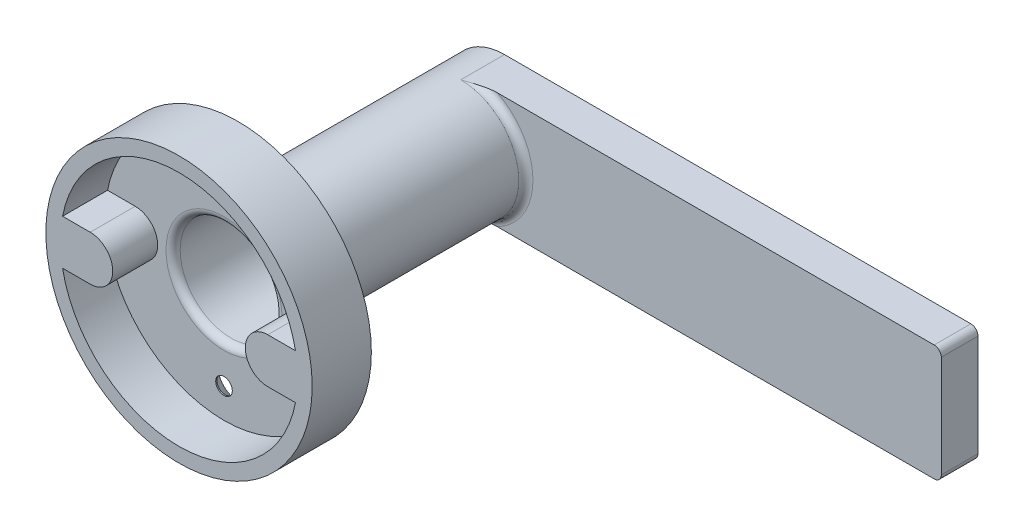
ISO-10303-21;
HEADER;
FILE_DESCRIPTION(('STEP AP214'),'2;1');
FILE_NAME('part.step','',(''),(''),'','','');
FILE_SCHEMA(('AUTOMOTIVE_DESIGN { 1 0 10303 214 1 1 1 1 }'));
ENDSEC;
DATA;
#1=APPLICATION_CONTEXT('core data for automotive mechanical design processes');
#2=APPLICATION_PROTOCOL_DEFINITION('international standard','automotive_design',2000,#1);
#3=PRODUCT_CONTEXT('',#1,'mechanical');
#4=PRODUCT('Part','Part','',(#3));
#5=PRODUCT_RELATED_PRODUCT_CATEGORY('part','',(#4));
#6=PRODUCT_DEFINITION_FORMATION('','',#4);
#7=PRODUCT_DEFINITION_CONTEXT('part definition',#1,'design');
#8=PRODUCT_DEFINITION('design','',#6,#7);
#9=PRODUCT_DEFINITION_SHAPE('','',#8);
#10=(LENGTH_UNIT() NAMED_UNIT(*) SI_UNIT(.MILLI.,.METRE.));
#11=(NAMED_UNIT(*) PLANE_ANGLE_UNIT() SI_UNIT($,.RADIAN.));
#12=(NAMED_UNIT(*) SI_UNIT($,.STERADIAN.) SOLID_ANGLE_UNIT());
#13=UNCERTAINTY_MEASURE_WITH_UNIT(LENGTH_MEASURE(1.E-05),#10,'distance_accuracy_value','');
#14=(GEOMETRIC_REPRESENTATION_CONTEXT(3) GLOBAL_UNCERTAINTY_ASSIGNED_CONTEXT((#13)) GLOBAL_UNIT_ASSIGNED_CONTEXT((#10,
#11,#12)) REPRESENTATION_CONTEXT('',''));
#15=CARTESIAN_POINT('',(0.,0.,0.));
#16=DIRECTION('',(0.,0.,1.));
#17=DIRECTION('',(1.,0.,0.));
#18=AXIS2_PLACEMENT_3D('',#15,#16,#17);
#19=CARTESIAN_POINT('',(0.,0.,12.7));
#20=DIRECTION('',(0.,0.,-1.));
#21=DIRECTION('',(-1.,0.,0.));
#22=AXIS2_PLACEMENT_3D('',#19,#20,#21);
#23=CYLINDRICAL_SURFACE('',#22,28.575);
#24=CARTESIAN_POINT('',(0.,0.,12.7));
#25=DIRECTION('',(0.,0.,1.));
#26=DIRECTION('',(1.,0.,0.));
#27=AXIS2_PLACEMENT_3D('',#24,#25,#26);
#28=CIRCLE('',#27,28.575);
#29=CARTESIAN_POINT('',(28.575,0.,12.7));
#30=VERTEX_POINT('',#29);
#31=EDGE_CURVE('E196',#30,#30,#28,.T.);
#32=ORIENTED_EDGE('',*,*,#31,.F.);
#33=EDGE_LOOP('',(#32));
#34=FACE_BOUND('',#33,.T.);
#35=CARTESIAN_POINT('',(0.,0.,0.));
#36=DIRECTION('',(0.,0.,1.));
#37=DIRECTION('',(1.,0.,0.));
#38=AXIS2_PLACEMENT_3D('',#35,#36,#37);
#39=CIRCLE('',#38,28.575);
#40=CARTESIAN_POINT('',(28.575,0.,0.));
#41=VERTEX_POINT('',#40);
#42=EDGE_CURVE('E247',#41,#41,#39,.T.);
#43=ORIENTED_EDGE('',*,*,#42,.T.);
#44=EDGE_LOOP('',(#43));
#45=FACE_BOUND('',#44,.T.);
#46=ADVANCED_FACE('F41',(#34,#45),#23,.T.);
#47=CARTESIAN_POINT('',(0.,0.,12.7));
#48=DIRECTION('',(0.,0.,1.));
#49=DIRECTION('',(1.,0.,0.));
#50=AXIS2_PLACEMENT_3D('',#47,#48,#49);
#51=PLANE('',#50);
#52=CARTESIAN_POINT('',(19.05,0.,12.7));
#53=DIRECTION('',(0.,0.,-1.));
#54=DIRECTION('',(-1.,0.,0.));
#55=AXIS2_PLACEMENT_3D('',#52,#53,#54);
#56=CIRCLE('',#55,4.826);
#57=CARTESIAN_POINT('',(19.05,-4.826,12.7));
#58=VERTEX_POINT('',#57);
#59=CARTESIAN_POINT('',(19.05,4.826,12.7));
#60=VERTEX_POINT('',#59);
#61=EDGE_CURVE('E195',#58,#60,#56,.T.);
#62=ORIENTED_EDGE('',*,*,#61,.F.);
#63=DIRECTION('',(-1.,0.,0.));
#64=VECTOR('',#63,1.);
#65=CARTESIAN_POINT('',(19.05,-4.826,12.7));
#66=LINE('',#65,#64);
#67=CARTESIAN_POINT('',(24.9900993985777,-4.826,12.7));
#68=VERTEX_POINT('',#67);
#69=EDGE_CURVE('E205',#68,#58,#66,.T.);
#70=ORIENTED_EDGE('',*,*,#69,.F.);
#71=CARTESIAN_POINT('',(0.,0.,12.7));
#72=DIRECTION('',(0.,0.,1.));
#73=DIRECTION('',(1.,0.,0.));
#74=AXIS2_PLACEMENT_3D('',#71,#72,#73);
#75=CIRCLE('',#74,25.451823980823);
#76=CARTESIAN_POINT('',(-24.9900993985777,-4.82599999999999,12.7));
#77=VERTEX_POINT('',#76);
#78=EDGE_CURVE('E241',#77,#68,#75,.T.);
#79=ORIENTED_EDGE('',*,*,#78,.F.);
#80=DIRECTION('',(-1.,0.,0.));
#81=VECTOR('',#80,1.);
#82=CARTESIAN_POINT('',(-19.05,-4.826,12.7));
#83=LINE('',#82,#81);
#84=CARTESIAN_POINT('',(-19.05,-4.826,12.7));
#85=VERTEX_POINT('',#84);
#86=EDGE_CURVE('E238',#85,#77,#83,.T.);
#87=ORIENTED_EDGE('',*,*,#86,.F.);
#88=CARTESIAN_POINT('',(-19.05,0.,12.7));
#89=DIRECTION('',(0.,0.,-1.));
#90=DIRECTION('',(1.,0.,0.));
#91=AXIS2_PLACEMENT_3D('',#88,#89,#90);
#92=CIRCLE('',#91,4.826);
#93=CARTESIAN_POINT('',(-19.05,4.826,12.7));
#94=VERTEX_POINT('',#93);
#95=EDGE_CURVE('E232',#94,#85,#92,.T.);
#96=ORIENTED_EDGE('',*,*,#95,.F.);
#97=DIRECTION('',(1.,0.,0.));
#98=VECTOR('',#97,1.);
#99=CARTESIAN_POINT('',(-19.05,4.826,12.7));
#100=LINE('',#99,#98);
#101=CARTESIAN_POINT('',(-24.9900993985777,4.826,12.7));
#102=VERTEX_POINT('',#101);
#103=EDGE_CURVE('E235',#102,#94,#100,.T.);
#104=ORIENTED_EDGE('',*,*,#103,.F.);
#105=CARTESIAN_POINT('',(0.,0.,12.7));
#106=DIRECTION('',(0.,0.,1.));
#107=DIRECTION('',(1.,0.,0.));
#108=AXIS2_PLACEMENT_3D('',#105,#106,#107);
#109=CIRCLE('',#108,25.451823980823);
#110=CARTESIAN_POINT('',(24.9900993985777,4.826,12.7));
#111=VERTEX_POINT('',#110);
#112=EDGE_CURVE('E230',#111,#102,#109,.T.);
#113=ORIENTED_EDGE('',*,*,#112,.F.);
#114=DIRECTION('',(1.,0.,0.));
#115=VECTOR('',#114,1.);
#116=CARTESIAN_POINT('',(19.05,4.826,12.7));
#117=LINE('',#116,#115);
#118=EDGE_CURVE('E228',#60,#111,#117,.T.);
#119=ORIENTED_EDGE('',*,*,#118,.F.);
#120=EDGE_LOOP('',(#62,#70,#79,#87,#96,#104,#113,#119));
#121=FACE_BOUND('',#120,.T.);
#122=ORIENTED_EDGE('',*,*,#31,.T.);
#123=EDGE_LOOP('',(#122));
#124=FACE_BOUND('',#123,.T.);
#125=ADVANCED_FACE('F342',(#121,#124),#51,.T.);
#126=CARTESIAN_POINT('',(0.,0.,0.));
#127=DIRECTION('',(0.,0.,1.));
#128=DIRECTION('',(1.,0.,0.));
#129=AXIS2_PLACEMENT_3D('',#126,#127,#128);
#130=PLANE('',#129);
#131=CARTESIAN_POINT('',(0.,-19.05,0.));
#132=DIRECTION('',(0.,0.,1.));
#133=DIRECTION('',(1.,0.,0.));
#134=AXIS2_PLACEMENT_3D('',#131,#132,#133);
#135=CIRCLE('',#134,4.37800000000003);
#136=CARTESIAN_POINT('',(4.37800000000003,-19.05,0.));
#137=VERTEX_POINT('',#136);
#138=EDGE_CURVE('E49',#137,#137,#135,.T.);
#139=ORIENTED_EDGE('',*,*,#138,.T.);
#140=EDGE_LOOP('',(#139));
#141=FACE_BOUND('',#140,.T.);
#142=CARTESIAN_POINT('',(0.,19.05,0.));
#143=DIRECTION('',(0.,0.,1.));
#144=DIRECTION('',(1.,0.,0.));
#145=AXIS2_PLACEMENT_3D('',#142,#143,#144);
#146=CIRCLE('',#145,4.37800000000003);
#147=CARTESIAN_POINT('',(4.37800000000003,19.05,0.));
#148=VERTEX_POINT('',#147);
#149=EDGE_CURVE('E425',#148,#148,#146,.T.);
#150=ORIENTED_EDGE('',*,*,#149,.T.);
#151=EDGE_LOOP('',(#150));
#152=FACE_BOUND('',#151,.T.);
#153=CARTESIAN_POINT('',(0.,0.,0.));
#154=DIRECTION('',(0.,0.,-1.));
#155=DIRECTION('',(-1.,0.,0.));
#156=AXIS2_PLACEMENT_3D('',#153,#154,#155);
#157=CIRCLE('',#156,12.446);
#158=CARTESIAN_POINT('',(-12.446,0.,0.));
#159=VERTEX_POINT('',#158);
#160=EDGE_CURVE('E193',#159,#159,#157,.T.);
#161=ORIENTED_EDGE('',*,*,#160,.F.);
#162=EDGE_LOOP('',(#161));
#163=FACE_BOUND('',#162,.T.);
#164=ORIENTED_EDGE('',*,*,#42,.F.);
#165=EDGE_LOOP('',(#164));
#166=FACE_BOUND('',#165,.T.);
#167=ADVANCED_FACE('F349',(#141,#152,#163,#166),#130,.F.);
#168=CARTESIAN_POINT('',(19.05,0.,3.048));
#169=DIRECTION('',(0.,0.,1.));
#170=DIRECTION('',(1.,0.,0.));
#171=AXIS2_PLACEMENT_3D('',#168,#169,#170);
#172=CYLINDRICAL_SURFACE('',#171,4.826);
#173=ORIENTED_EDGE('',*,*,#61,.T.);
#174=DIRECTION('',(0.,0.,1.));
#175=VECTOR('',#174,1.);
#176=CARTESIAN_POINT('',(19.05,4.826,3.048));
#177=LINE('',#176,#175);
#178=CARTESIAN_POINT('',(19.05,4.826,3.048));
#179=VERTEX_POINT('',#178);
#180=EDGE_CURVE('E221',#179,#60,#177,.T.);
#181=ORIENTED_EDGE('',*,*,#180,.F.);
#182=CARTESIAN_POINT('',(19.05,0.,3.048));
#183=DIRECTION('',(0.,0.,-1.));
#184=DIRECTION('',(-1.,0.,0.));
#185=AXIS2_PLACEMENT_3D('',#182,#183,#184);
#186=CIRCLE('',#185,4.826);
#187=CARTESIAN_POINT('',(19.05,-4.826,3.048));
#188=VERTEX_POINT('',#187);
#189=EDGE_CURVE('E197',#188,#179,#186,.T.);
#190=ORIENTED_EDGE('',*,*,#189,.F.);
#191=DIRECTION('',(0.,0.,1.));
#192=VECTOR('',#191,1.);
#193=CARTESIAN_POINT('',(19.05,-4.826,3.048));
#194=LINE('',#193,#192);
#195=EDGE_CURVE('E246',#188,#58,#194,.T.);
#196=ORIENTED_EDGE('',*,*,#195,.T.);
#197=EDGE_LOOP('',(#173,#181,#190,#196));
#198=FACE_BOUND('',#197,.T.);
#199=ADVANCED_FACE('F356',(#198),#172,.T.);
#200=CARTESIAN_POINT('',(19.05,-4.826,3.048));
#201=DIRECTION('',(0.,1.,0.));
#202=DIRECTION('',(-1.,0.,0.));
#203=AXIS2_PLACEMENT_3D('',#200,#201,#202);
#204=PLANE('',#203);
#205=ORIENTED_EDGE('',*,*,#69,.T.);
#206=ORIENTED_EDGE('',*,*,#195,.F.);
#207=DIRECTION('',(-1.,0.,0.));
#208=VECTOR('',#207,1.);
#209=CARTESIAN_POINT('',(19.05,-4.826,3.048));
#210=LINE('',#209,#208);
#211=CARTESIAN_POINT('',(24.9900993985777,-4.826,3.048));
#212=VERTEX_POINT('',#211);
#213=EDGE_CURVE('E222',#212,#188,#210,.T.);
#214=ORIENTED_EDGE('',*,*,#213,.F.);
#215=DIRECTION('',(0.,0.,1.));
#216=VECTOR('',#215,1.);
#217=CARTESIAN_POINT('',(24.9900993985777,-4.826,3.048));
#218=LINE('',#217,#216);
#219=EDGE_CURVE('E248',#212,#68,#218,.T.);
#220=ORIENTED_EDGE('',*,*,#219,.T.);
#221=EDGE_LOOP('',(#205,#206,#214,#220));
#222=FACE_BOUND('',#221,.T.);
#223=ADVANCED_FACE('F362',(#222),#204,.F.);
#224=CARTESIAN_POINT('',(0.,0.,3.048));
#225=DIRECTION('',(0.,0.,1.));
#226=DIRECTION('',(1.,0.,0.));
#227=AXIS2_PLACEMENT_3D('',#224,#225,#226);
#228=CYLINDRICAL_SURFACE('',#227,25.451823980823);
#229=ORIENTED_EDGE('',*,*,#78,.T.);
#230=ORIENTED_EDGE('',*,*,#219,.F.);
#231=CARTESIAN_POINT('',(0.,0.,3.048));
#232=DIRECTION('',(0.,0.,1.));
#233=DIRECTION('',(1.,0.,0.));
#234=AXIS2_PLACEMENT_3D('',#231,#232,#233);
#235=CIRCLE('',#234,25.451823980823);
#236=CARTESIAN_POINT('',(-24.9900993985777,-4.82599999999999,3.048));
#237=VERTEX_POINT('',#236);
#238=EDGE_CURVE('E216',#237,#212,#235,.T.);
#239=ORIENTED_EDGE('',*,*,#238,.F.);
#240=DIRECTION('',(0.,0.,1.));
#241=VECTOR('',#240,1.);
#242=CARTESIAN_POINT('',(-24.9900993985777,-4.82599999999999,3.048));
#243=LINE('',#242,#241);
#244=EDGE_CURVE('E252',#237,#77,#243,.T.);
#245=ORIENTED_EDGE('',*,*,#244,.T.);
#246=EDGE_LOOP('',(#229,#230,#239,#245));
#247=FACE_BOUND('',#246,.T.);
#248=ADVANCED_FACE('F393',(#247),#228,.F.);
#249=CARTESIAN_POINT('',(-19.05,-4.826,3.048));
#250=DIRECTION('',(0.,1.,0.));
#251=DIRECTION('',(-1.,0.,0.));
#252=AXIS2_PLACEMENT_3D('',#249,#250,#251);
#253=PLANE('',#252);
#254=ORIENTED_EDGE('',*,*,#86,.T.);
#255=ORIENTED_EDGE('',*,*,#244,.F.);
#256=DIRECTION('',(-1.,0.,0.));
#257=VECTOR('',#256,1.);
#258=CARTESIAN_POINT('',(-19.05,-4.826,3.048));
#259=LINE('',#258,#257);
#260=CARTESIAN_POINT('',(-19.05,-4.826,3.048));
#261=VERTEX_POINT('',#260);
#262=EDGE_CURVE('E212',#261,#237,#259,.T.);
#263=ORIENTED_EDGE('',*,*,#262,.F.);
#264=DIRECTION('',(0.,0.,1.));
#265=VECTOR('',#264,1.);
#266=CARTESIAN_POINT('',(-19.05,-4.826,3.048));
#267=LINE('',#266,#265);
#268=EDGE_CURVE('E254',#261,#85,#267,.T.);
#269=ORIENTED_EDGE('',*,*,#268,.T.);
#270=EDGE_LOOP('',(#254,#255,#263,#269));
#271=FACE_BOUND('',#270,.T.);
#272=ADVANCED_FACE('F386',(#271),#253,.F.);
#273=CARTESIAN_POINT('',(-19.05,0.,3.048));
#274=DIRECTION('',(0.,0.,1.));
#275=DIRECTION('',(1.,0.,0.));
#276=AXIS2_PLACEMENT_3D('',#273,#274,#275);
#277=CYLINDRICAL_SURFACE('',#276,4.826);
#278=ORIENTED_EDGE('',*,*,#95,.T.);
#279=ORIENTED_EDGE('',*,*,#268,.F.);
#280=CARTESIAN_POINT('',(-19.05,0.,3.048));
#281=DIRECTION('',(0.,0.,-1.));
#282=DIRECTION('',(1.,0.,0.));
#283=AXIS2_PLACEMENT_3D('',#280,#281,#282);
#284=CIRCLE('',#283,4.826);
#285=CARTESIAN_POINT('',(-19.05,4.826,3.048));
#286=VERTEX_POINT('',#285);
#287=EDGE_CURVE('E211',#286,#261,#284,.T.);
#288=ORIENTED_EDGE('',*,*,#287,.F.);
#289=DIRECTION('',(0.,0.,1.));
#290=VECTOR('',#289,1.);
#291=CARTESIAN_POINT('',(-19.05,4.826,3.048));
#292=LINE('',#291,#290);
#293=EDGE_CURVE('E253',#286,#94,#292,.T.);
#294=ORIENTED_EDGE('',*,*,#293,.T.);
#295=EDGE_LOOP('',(#278,#279,#288,#294));
#296=FACE_BOUND('',#295,.T.);
#297=ADVANCED_FACE('F384',(#296),#277,.T.);
#298=CARTESIAN_POINT('',(-19.05,4.826,3.048));
#299=DIRECTION('',(0.,-1.,0.));
#300=DIRECTION('',(1.,0.,0.));
#301=AXIS2_PLACEMENT_3D('',#298,#299,#300);
#302=PLANE('',#301);
#303=ORIENTED_EDGE('',*,*,#103,.T.);
#304=ORIENTED_EDGE('',*,*,#293,.F.);
#305=DIRECTION('',(1.,0.,0.));
#306=VECTOR('',#305,1.);
#307=CARTESIAN_POINT('',(-19.05,4.826,3.048));
#308=LINE('',#307,#306);
#309=CARTESIAN_POINT('',(-24.9900993985777,4.826,3.048));
#310=VERTEX_POINT('',#309);
#311=EDGE_CURVE('E209',#310,#286,#308,.T.);
#312=ORIENTED_EDGE('',*,*,#311,.F.);
#313=DIRECTION('',(0.,0.,1.));
#314=VECTOR('',#313,1.);
#315=CARTESIAN_POINT('',(-24.9900993985777,4.826,3.048));
#316=LINE('',#315,#314);
#317=EDGE_CURVE('E256',#310,#102,#316,.T.);
#318=ORIENTED_EDGE('',*,*,#317,.T.);
#319=EDGE_LOOP('',(#303,#304,#312,#318));
#320=FACE_BOUND('',#319,.T.);
#321=ADVANCED_FACE('F378',(#320),#302,.F.);
#322=CARTESIAN_POINT('',(0.,0.,3.048));
#323=DIRECTION('',(0.,0.,1.));
#324=DIRECTION('',(1.,0.,0.));
#325=AXIS2_PLACEMENT_3D('',#322,#323,#324);
#326=CYLINDRICAL_SURFACE('',#325,25.451823980823);
#327=ORIENTED_EDGE('',*,*,#112,.T.);
#328=ORIENTED_EDGE('',*,*,#317,.F.);
#329=CARTESIAN_POINT('',(0.,0.,3.048));
#330=DIRECTION('',(0.,0.,1.));
#331=DIRECTION('',(1.,0.,0.));
#332=AXIS2_PLACEMENT_3D('',#329,#330,#331);
#333=CIRCLE('',#332,25.451823980823);
#334=CARTESIAN_POINT('',(24.9900993985777,4.826,3.048));
#335=VERTEX_POINT('',#334);
#336=EDGE_CURVE('E207',#335,#310,#333,.T.);
#337=ORIENTED_EDGE('',*,*,#336,.F.);
#338=DIRECTION('',(0.,0.,1.));
#339=VECTOR('',#338,1.);
#340=CARTESIAN_POINT('',(24.9900993985777,4.826,3.048));
#341=LINE('',#340,#339);
#342=EDGE_CURVE('E258',#335,#111,#341,.T.);
#343=ORIENTED_EDGE('',*,*,#342,.T.);
#344=EDGE_LOOP('',(#327,#328,#337,#343));
#345=FACE_BOUND('',#344,.T.);
#346=ADVANCED_FACE('F374',(#345),#326,.F.);
#347=CARTESIAN_POINT('',(19.05,4.826,3.048));
#348=DIRECTION('',(0.,-1.,0.));
#349=DIRECTION('',(1.,0.,0.));
#350=AXIS2_PLACEMENT_3D('',#347,#348,#349);
#351=PLANE('',#350);
#352=ORIENTED_EDGE('',*,*,#118,.T.);
#353=ORIENTED_EDGE('',*,*,#342,.F.);
#354=DIRECTION('',(1.,0.,0.));
#355=VECTOR('',#354,1.);
#356=CARTESIAN_POINT('',(19.05,4.826,3.048));
#357=LINE('',#356,#355);
#358=EDGE_CURVE('E204',#179,#335,#357,.T.);
#359=ORIENTED_EDGE('',*,*,#358,.F.);
#360=ORIENTED_EDGE('',*,*,#180,.T.);
#361=EDGE_LOOP('',(#352,#353,#359,#360));
#362=FACE_BOUND('',#361,.T.);
#363=ADVANCED_FACE('F371',(#362),#351,.F.);
#364=CARTESIAN_POINT('',(19.05,0.,3.048));
#365=DIRECTION('',(0.,0.,-1.));
#366=DIRECTION('',(-1.,0.,0.));
#367=AXIS2_PLACEMENT_3D('',#364,#365,#366);
#368=PLANE('',#367);
#369=CARTESIAN_POINT('',(0.,19.05,3.048));
#370=DIRECTION('',(0.,0.,1.));
#371=DIRECTION('',(1.,0.,0.));
#372=AXIS2_PLACEMENT_3D('',#369,#370,#371);
#373=CIRCLE('',#372,1.778);
#374=CARTESIAN_POINT('',(1.778,19.05,3.048));
#375=VERTEX_POINT('',#374);
#376=EDGE_CURVE('E187',#375,#375,#373,.T.);
#377=ORIENTED_EDGE('',*,*,#376,.F.);
#378=EDGE_LOOP('',(#377));
#379=FACE_BOUND('',#378,.T.);
#380=CARTESIAN_POINT('',(0.,-19.05,3.048));
#381=DIRECTION('',(0.,0.,1.));
#382=DIRECTION('',(-1.,0.,0.));
#383=AXIS2_PLACEMENT_3D('',#380,#381,#382);
#384=CIRCLE('',#383,1.778);
#385=CARTESIAN_POINT('',(-1.778,-19.05,3.048));
#386=VERTEX_POINT('',#385);
#387=EDGE_CURVE('E436',#386,#386,#384,.T.);
#388=ORIENTED_EDGE('',*,*,#387,.F.);
#389=EDGE_LOOP('',(#388));
#390=FACE_BOUND('',#389,.T.);
#391=CARTESIAN_POINT('',(0.,0.,3.048));
#392=DIRECTION('',(0.,0.,-1.));
#393=DIRECTION('',(-1.,0.,0.));
#394=AXIS2_PLACEMENT_3D('',#391,#392,#393);
#395=CIRCLE('',#394,12.446);
#396=CARTESIAN_POINT('',(-12.446,0.,3.048));
#397=VERTEX_POINT('',#396);
#398=EDGE_CURVE('E280',#397,#397,#395,.T.);
#399=ORIENTED_EDGE('',*,*,#398,.T.);
#400=EDGE_LOOP('',(#399));
#401=FACE_BOUND('',#400,.T.);
#402=ORIENTED_EDGE('',*,*,#189,.T.);
#403=ORIENTED_EDGE('',*,*,#358,.T.);
#404=ORIENTED_EDGE('',*,*,#336,.T.);
#405=ORIENTED_EDGE('',*,*,#311,.T.);
#406=ORIENTED_EDGE('',*,*,#287,.T.);
#407=ORIENTED_EDGE('',*,*,#262,.T.);
#408=ORIENTED_EDGE('',*,*,#238,.T.);
#409=ORIENTED_EDGE('',*,*,#213,.T.);
#410=EDGE_LOOP('',(#402,#403,#404,#405,#406,#407,#408,#409));
#411=FACE_BOUND('',#410,.T.);
#412=ADVANCED_FACE('F372',(#379,#390,#401,#411),#368,.F.);
#413=CARTESIAN_POINT('',(0.,0.,-49.276));
#414=DIRECTION('',(0.,0.,1.));
#415=DIRECTION('',(1.,0.,0.));
#416=AXIS2_PLACEMENT_3D('',#413,#414,#415);
#417=CYLINDRICAL_SURFACE('',#416,12.446);
#418=DIRECTION('',(0.,0.,1.));
#419=VECTOR('',#418,1.);
#420=CARTESIAN_POINT('',(0.,-12.446,-57.15));
#421=LINE('',#420,#419);
#422=CARTESIAN_POINT('',(0.,-12.446,-57.15));
#423=VERTEX_POINT('',#422);
#424=CARTESIAN_POINT('',(0.,-12.446,-47.752));
#425=VERTEX_POINT('',#424);
#426=EDGE_CURVE('E168',#423,#425,#421,.T.);
#427=ORIENTED_EDGE('',*,*,#426,.T.);
#428=CARTESIAN_POINT('',(0.,0.,-47.752));
#429=DIRECTION('',(0.,0.,-1.));
#430=DIRECTION('',(-1.,0.,0.));
#431=AXIS2_PLACEMENT_3D('',#428,#429,#430);
#432=CIRCLE('',#431,12.446);
#433=CARTESIAN_POINT('',(0.,12.446,-47.752));
#434=VERTEX_POINT('',#433);
#435=EDGE_CURVE('E271',#425,#434,#432,.F.);
#436=ORIENTED_EDGE('',*,*,#435,.T.);
#437=DIRECTION('',(0.,0.,1.));
#438=VECTOR('',#437,1.);
#439=CARTESIAN_POINT('',(0.,12.446,-57.15));
#440=LINE('',#439,#438);
#441=CARTESIAN_POINT('',(0.,12.446,-57.15));
#442=VERTEX_POINT('',#441);
#443=EDGE_CURVE('E172',#442,#434,#440,.T.);
#444=ORIENTED_EDGE('',*,*,#443,.F.);
#445=CARTESIAN_POINT('',(0.,0.,-57.15));
#446=DIRECTION('',(0.,0.,-1.));
#447=DIRECTION('',(-1.,0.,0.));
#448=AXIS2_PLACEMENT_3D('',#445,#446,#447);
#449=CIRCLE('',#448,12.446);
#450=EDGE_CURVE('E157',#423,#442,#449,.T.);
#451=ORIENTED_EDGE('',*,*,#450,.F.);
#452=EDGE_LOOP('',(#427,#436,#444,#451));
#453=FACE_BOUND('',#452,.T.);
#454=ORIENTED_EDGE('',*,*,#160,.T.);
#455=EDGE_LOOP('',(#454));
#456=FACE_BOUND('',#455,.T.);
#457=ADVANCED_FACE('F176',(#453,#456),#417,.T.);
#458=CARTESIAN_POINT('',(0.,0.,-80.1680810564779));
#459=DIRECTION('',(0.,0.,1.));
#460=DIRECTION('',(1.,0.,0.));
#461=AXIS2_PLACEMENT_3D('',#458,#459,#460);
#462=CYLINDRICAL_SURFACE('',#461,10.922);
#463=CARTESIAN_POINT('',(0.,0.,1.524));
#464=DIRECTION('',(0.,0.,-1.));
#465=DIRECTION('',(-1.,0.,0.));
#466=AXIS2_PLACEMENT_3D('',#463,#464,#465);
#467=CIRCLE('',#466,10.922);
#468=CARTESIAN_POINT('',(-10.922,0.,1.524));
#469=VERTEX_POINT('',#468);
#470=EDGE_CURVE('E273',#469,#469,#467,.F.);
#471=ORIENTED_EDGE('',*,*,#470,.T.);
#472=EDGE_LOOP('',(#471));
#473=FACE_BOUND('',#472,.T.);
#474=CARTESIAN_POINT('',(0.,0.,-49.276));
#475=DIRECTION('',(0.,0.,-1.));
#476=DIRECTION('',(-1.,0.,0.));
#477=AXIS2_PLACEMENT_3D('',#474,#475,#476);
#478=CIRCLE('',#477,10.922);
#479=CARTESIAN_POINT('',(-10.922,0.,-49.276));
#480=VERTEX_POINT('',#479);
#481=EDGE_CURVE('E173',#480,#480,#478,.F.);
#482=ORIENTED_EDGE('',*,*,#481,.F.);
#483=EDGE_LOOP('',(#482));
#484=FACE_BOUND('',#483,.T.);
#485=ADVANCED_FACE('F401',(#473,#484),#462,.F.);
#486=CARTESIAN_POINT('',(0.,0.,-57.15));
#487=DIRECTION('',(0.,0.,-1.));
#488=DIRECTION('',(-1.,0.,0.));
#489=AXIS2_PLACEMENT_3D('',#486,#487,#488);
#490=PLANE('',#489);
#491=DIRECTION('',(0.,-1.,0.));
#492=VECTOR('',#491,1.);
#493=CARTESIAN_POINT('',(101.6,12.446,-57.15));
#494=LINE('',#493,#492);
#495=CARTESIAN_POINT('',(101.6,10.922,-57.15));
#496=VERTEX_POINT('',#495);
#497=CARTESIAN_POINT('',(101.6,-10.922,-57.15));
#498=VERTEX_POINT('',#497);
#499=EDGE_CURVE('E161',#496,#498,#494,.T.);
#500=ORIENTED_EDGE('',*,*,#499,.T.);
#501=CARTESIAN_POINT('',(100.076,-10.922,-57.15));
#502=DIRECTION('',(0.,0.,-1.));
#503=DIRECTION('',(-1.,0.,0.));
#504=AXIS2_PLACEMENT_3D('',#501,#502,#503);
#505=CIRCLE('',#504,1.524);
#506=CARTESIAN_POINT('',(100.076,-12.446,-57.15));
#507=VERTEX_POINT('',#506);
#508=EDGE_CURVE('E156',#498,#507,#505,.T.);
#509=ORIENTED_EDGE('',*,*,#508,.T.);
#510=DIRECTION('',(-1.,0.,0.));
#511=VECTOR('',#510,1.);
#512=CARTESIAN_POINT('',(101.6,-12.446,-57.15));
#513=LINE('',#512,#511);
#514=EDGE_CURVE('E155',#507,#423,#513,.T.);
#515=ORIENTED_EDGE('',*,*,#514,.T.);
#516=ORIENTED_EDGE('',*,*,#450,.T.);
#517=DIRECTION('',(1.,0.,0.));
#518=VECTOR('',#517,1.);
#519=CARTESIAN_POINT('',(101.6,12.446,-57.15));
#520=LINE('',#519,#518);
#521=CARTESIAN_POINT('',(100.076,12.446,-57.15));
#522=VERTEX_POINT('',#521);
#523=EDGE_CURVE('E178',#442,#522,#520,.T.);
#524=ORIENTED_EDGE('',*,*,#523,.T.);
#525=CARTESIAN_POINT('',(100.076,10.922,-57.15));
#526=DIRECTION('',(0.,0.,-1.));
#527=DIRECTION('',(-1.,0.,0.));
#528=AXIS2_PLACEMENT_3D('',#525,#526,#527);
#529=CIRCLE('',#528,1.524);
#530=EDGE_CURVE('E289',#522,#496,#529,.T.);
#531=ORIENTED_EDGE('',*,*,#530,.T.);
#532=EDGE_LOOP('',(#500,#509,#515,#516,#524,#531));
#533=FACE_BOUND('',#532,.T.);
#534=ADVANCED_FACE('F152',(#533),#490,.T.);
#535=CARTESIAN_POINT('',(101.6,12.446,-57.15));
#536=DIRECTION('',(0.,-1.,0.));
#537=DIRECTION('',(0.,0.,-1.));
#538=AXIS2_PLACEMENT_3D('',#535,#536,#537);
#539=PLANE('',#538);
#540=DIRECTION('',(1.,0.,0.));
#541=VECTOR('',#540,1.);
#542=CARTESIAN_POINT('',(101.6,12.446,-49.276));
#543=LINE('',#542,#541);
#544=CARTESIAN_POINT('',(6.34491796637277,12.446,-49.276));
#545=VERTEX_POINT('',#544);
#546=CARTESIAN_POINT('',(100.076,12.446,-49.276));
#547=VERTEX_POINT('',#546);
#548=EDGE_CURVE('E189',#545,#547,#543,.T.);
#549=ORIENTED_EDGE('',*,*,#548,.T.);
#550=DIRECTION('',(0.,0.,1.));
#551=VECTOR('',#550,1.);
#552=CARTESIAN_POINT('',(100.076,12.446,-57.15));
#553=LINE('',#552,#551);
#554=EDGE_CURVE('E60',#547,#522,#553,.F.);
#555=ORIENTED_EDGE('',*,*,#554,.T.);
#556=ORIENTED_EDGE('',*,*,#523,.F.);
#557=ORIENTED_EDGE('',*,*,#443,.T.);
#558=CARTESIAN_POINT('',(6.34491796637277,12.446,-49.276));
#559=CARTESIAN_POINT('',(6.21533524094485,12.446,-49.2759732705405));
#560=CARTESIAN_POINT('',(6.08579369063811,12.446,-49.27259226928));
#561=CARTESIAN_POINT('',(5.82706524459241,12.446,-49.259910087951));
#562=CARTESIAN_POINT('',(5.6978781945778,12.446,-49.2506121205866));
#563=CARTESIAN_POINT('',(5.4402955593906,12.446,-49.2269107528351));
#564=CARTESIAN_POINT('',(5.31189882415412,12.446,-49.2125195023357));
#565=CARTESIAN_POINT('',(5.05567590714475,12.446,-49.1792496205522));
#566=CARTESIAN_POINT('',(4.92784981517291,12.446,-49.1603703067066));
#567=CARTESIAN_POINT('',(4.54726190236325,12.446,-49.0981575716032));
#568=CARTESIAN_POINT('',(4.29543863295937,12.446,-49.0490520465874));
#569=CARTESIAN_POINT('',(3.79431096207436,12.446,-48.9389015359754));
#570=CARTESIAN_POINT('',(3.54500841851374,12.446,-48.8778483354951));
#571=CARTESIAN_POINT('',(3.01979635859548,12.446,-48.7389881468602));
#572=CARTESIAN_POINT('',(2.74418711385954,12.446,-48.6600566773526));
#573=CARTESIAN_POINT('',(2.19547772469525,12.446,-48.4941969315973));
#574=CARTESIAN_POINT('',(1.92237711929461,12.446,-48.4072701582111));
#575=CARTESIAN_POINT('',(1.1047936535399,12.446,-48.1385183371954));
#576=CARTESIAN_POINT('',(0.562885676700975,12.446,-47.9489679517187));
#577=CARTESIAN_POINT('',(0.0140400977837042,12.446,-47.7569129993086));
#578=CARTESIAN_POINT('',(0.00702004561032453,12.446,-47.7544564925513));
#579=CARTESIAN_POINT('',(0.,12.446,-47.752));
#580=B_SPLINE_CURVE_WITH_KNOTS('',3,(#558,#559,#560,#561,#562,#563,#564,#565,#566,#567,#568,
#569,#570,#571,#572,#573,#574,#575,#576,#577,#578,#579),.UNSPECIFIED.,.F.,.F.,(4,2,2,2,2,2,2,2,
2,2,4),(0.,0.388645930924585,0.777081020636638,1.16459568621553,1.5521693242234,
2.32144242636155,3.09124632924267,3.95113147757733,4.81085532404043,6.5329742853189,
6.5552866137498),.UNSPECIFIED.);
#581=EDGE_CURVE('E296',#434,#545,#580,.F.);
#582=ORIENTED_EDGE('',*,*,#581,.T.);
#583=EDGE_LOOP('',(#549,#555,#556,#557,#582));
#584=FACE_BOUND('',#583,.T.);
#585=ADVANCED_FACE('F414',(#584),#539,.F.);
#586=CARTESIAN_POINT('',(101.6,-12.446,-57.15));
#587=DIRECTION('',(0.,1.,0.));
#588=DIRECTION('',(0.,0.,1.));
#589=AXIS2_PLACEMENT_3D('',#586,#587,#588);
#590=PLANE('',#589);
#591=ORIENTED_EDGE('',*,*,#514,.F.);
#592=DIRECTION('',(0.,0.,1.));
#593=VECTOR('',#592,1.);
#594=CARTESIAN_POINT('',(100.076,-12.446,-57.15));
#595=LINE('',#594,#593);
#596=CARTESIAN_POINT('',(100.076,-12.446,-49.276));
#597=VERTEX_POINT('',#596);
#598=EDGE_CURVE('E283',#507,#597,#595,.T.);
#599=ORIENTED_EDGE('',*,*,#598,.T.);
#600=DIRECTION('',(-1.,0.,0.));
#601=VECTOR('',#600,1.);
#602=CARTESIAN_POINT('',(101.6,-12.446,-49.276));
#603=LINE('',#602,#601);
#604=CARTESIAN_POINT('',(6.34491796637277,-12.446,-49.276));
#605=VERTEX_POINT('',#604);
#606=EDGE_CURVE('E184',#597,#605,#603,.T.);
#607=ORIENTED_EDGE('',*,*,#606,.T.);
#608=CARTESIAN_POINT('',(6.34491796637277,-12.446,-49.276));
#609=CARTESIAN_POINT('',(6.21533524094485,-12.446,-49.2759732705405));
#610=CARTESIAN_POINT('',(6.08579369063811,-12.446,-49.27259226928));
#611=CARTESIAN_POINT('',(5.82706524459241,-12.446,-49.259910087951));
#612=CARTESIAN_POINT('',(5.6978781945778,-12.446,-49.2506121205866));
#613=CARTESIAN_POINT('',(5.4402955593906,-12.446,-49.2269107528351));
#614=CARTESIAN_POINT('',(5.31189882415412,-12.446,-49.2125195023357));
#615=CARTESIAN_POINT('',(5.05567590714475,-12.446,-49.1792496205522));
#616=CARTESIAN_POINT('',(4.92784981517291,-12.446,-49.1603703067066));
#617=CARTESIAN_POINT('',(4.54726190236325,-12.446,-49.0981575716032));
#618=CARTESIAN_POINT('',(4.29543863295937,-12.446,-49.0490520465874));
#619=CARTESIAN_POINT('',(3.79431096207436,-12.446,-48.9389015359754));
#620=CARTESIAN_POINT('',(3.54500841851374,-12.446,-48.8778483354951));
#621=CARTESIAN_POINT('',(3.01979635859548,-12.446,-48.7389881468602));
#622=CARTESIAN_POINT('',(2.74418711385954,-12.446,-48.6600566773526));
#623=CARTESIAN_POINT('',(2.19547772469525,-12.446,-48.4941969315973));
#624=CARTESIAN_POINT('',(1.92237711929461,-12.446,-48.4072701582111));
#625=CARTESIAN_POINT('',(1.1047936535399,-12.446,-48.1385183371954));
#626=CARTESIAN_POINT('',(0.562885676700975,-12.446,-47.9489679517187));
#627=CARTESIAN_POINT('',(0.0140400977837042,-12.446,-47.7569129993086));
#628=CARTESIAN_POINT('',(0.00702004561032453,-12.446,-47.7544564925513));
#629=CARTESIAN_POINT('',(0.,-12.446,-47.752));
#630=B_SPLINE_CURVE_WITH_KNOTS('',3,(#608,#609,#610,#611,#612,#613,#614,#615,#616,#617,#618,
#619,#620,#621,#622,#623,#624,#625,#626,#627,#628,#629),.UNSPECIFIED.,.F.,.F.,(4,2,2,2,2,2,2,2,
2,2,4),(0.,0.388645930924585,0.777081020636638,1.16459568621553,1.5521693242234,
2.32144242636155,3.09124632924267,3.95113147757733,4.81085532404043,6.5329742853189,
6.5552866137498),.UNSPECIFIED.);
#631=EDGE_CURVE('E169',#605,#425,#630,.T.);
#632=ORIENTED_EDGE('',*,*,#631,.T.);
#633=ORIENTED_EDGE('',*,*,#426,.F.);
#634=EDGE_LOOP('',(#591,#599,#607,#632,#633));
#635=FACE_BOUND('',#634,.T.);
#636=ADVANCED_FACE('F170',(#635),#590,.F.);
#637=CARTESIAN_POINT('',(101.6,12.446,-57.15));
#638=DIRECTION('',(-1.,0.,0.));
#639=DIRECTION('',(0.,0.,1.));
#640=AXIS2_PLACEMENT_3D('',#637,#638,#639);
#641=PLANE('',#640);
#642=DIRECTION('',(0.,-1.,0.));
#643=VECTOR('',#642,1.);
#644=CARTESIAN_POINT('',(101.6,12.446,-49.276));
#645=LINE('',#644,#643);
#646=CARTESIAN_POINT('',(101.6,10.922,-49.276));
#647=VERTEX_POINT('',#646);
#648=CARTESIAN_POINT('',(101.6,-10.922,-49.276));
#649=VERTEX_POINT('',#648);
#650=EDGE_CURVE('E182',#647,#649,#645,.T.);
#651=ORIENTED_EDGE('',*,*,#650,.T.);
#652=DIRECTION('',(0.,0.,1.));
#653=VECTOR('',#652,1.);
#654=CARTESIAN_POINT('',(101.6,-10.922,-57.15));
#655=LINE('',#654,#653);
#656=EDGE_CURVE('E62',#649,#498,#655,.F.);
#657=ORIENTED_EDGE('',*,*,#656,.T.);
#658=ORIENTED_EDGE('',*,*,#499,.F.);
#659=DIRECTION('',(0.,0.,1.));
#660=VECTOR('',#659,1.);
#661=CARTESIAN_POINT('',(101.6,10.922,-57.15));
#662=LINE('',#661,#660);
#663=EDGE_CURVE('E281',#496,#647,#662,.T.);
#664=ORIENTED_EDGE('',*,*,#663,.T.);
#665=EDGE_LOOP('',(#651,#657,#658,#664));
#666=FACE_BOUND('',#665,.T.);
#667=ADVANCED_FACE('F409',(#666),#641,.F.);
#668=CARTESIAN_POINT('',(0.,0.,-49.276));
#669=DIRECTION('',(0.,0.,-1.));
#670=DIRECTION('',(-1.,0.,0.));
#671=AXIS2_PLACEMENT_3D('',#668,#669,#670);
#672=PLANE('',#671);
#673=ORIENTED_EDGE('',*,*,#548,.F.);
#674=CARTESIAN_POINT('',(0.,0.,-49.276));
#675=DIRECTION('',(0.,0.,-1.));
#676=DIRECTION('',(-1.,0.,0.));
#677=AXIS2_PLACEMENT_3D('',#674,#675,#676);
#678=CIRCLE('',#677,13.97);
#679=EDGE_CURVE('E268',#545,#605,#678,.T.);
#680=ORIENTED_EDGE('',*,*,#679,.T.);
#681=ORIENTED_EDGE('',*,*,#606,.F.);
#682=CARTESIAN_POINT('',(100.076,-10.922,-49.276));
#683=DIRECTION('',(0.,0.,-1.));
#684=DIRECTION('',(-1.,0.,0.));
#685=AXIS2_PLACEMENT_3D('',#682,#683,#684);
#686=CIRCLE('',#685,1.524);
#687=EDGE_CURVE('E270',#597,#649,#686,.F.);
#688=ORIENTED_EDGE('',*,*,#687,.T.);
#689=ORIENTED_EDGE('',*,*,#650,.F.);
#690=CARTESIAN_POINT('',(100.076,10.922,-49.276));
#691=DIRECTION('',(0.,0.,-1.));
#692=DIRECTION('',(-1.,0.,0.));
#693=AXIS2_PLACEMENT_3D('',#690,#691,#692);
#694=CIRCLE('',#693,1.524);
#695=EDGE_CURVE('E200',#647,#547,#694,.F.);
#696=ORIENTED_EDGE('',*,*,#695,.T.);
#697=EDGE_LOOP('',(#673,#680,#681,#688,#689,#696));
#698=FACE_BOUND('',#697,.T.);
#699=ADVANCED_FACE('F410',(#698),#672,.F.);
#700=ORIENTED_EDGE('',*,*,#481,.T.);
#701=EDGE_LOOP('',(#700));
#702=FACE_BOUND('',#701,.T.);
#703=ADVANCED_FACE('F312',(#702),#672,.F.);
#704=CARTESIAN_POINT('',(0.,0.,-47.752));
#705=DIRECTION('',(0.,0.,-1.));
#706=DIRECTION('',(-1.,0.,0.));
#707=AXIS2_PLACEMENT_3D('',#704,#705,#706);
#708=TOROIDAL_SURFACE('',#707,13.97,1.524);
#709=ORIENTED_EDGE('',*,*,#581,.F.);
#710=ORIENTED_EDGE('',*,*,#435,.F.);
#711=ORIENTED_EDGE('',*,*,#631,.F.);
#712=ORIENTED_EDGE('',*,*,#679,.F.);
#713=EDGE_LOOP('',(#709,#710,#711,#712));
#714=FACE_BOUND('',#713,.T.);
#715=ADVANCED_FACE('F310',(#714),#708,.F.);
#716=CARTESIAN_POINT('',(0.,0.,1.524));
#717=DIRECTION('',(0.,0.,-1.));
#718=DIRECTION('',(-1.,0.,0.));
#719=AXIS2_PLACEMENT_3D('',#716,#717,#718);
#720=TOROIDAL_SURFACE('',#719,12.446,1.524);
#721=ORIENTED_EDGE('',*,*,#398,.F.);
#722=EDGE_LOOP('',(#721));
#723=FACE_BOUND('',#722,.T.);
#724=ORIENTED_EDGE('',*,*,#470,.F.);
#725=EDGE_LOOP('',(#724));
#726=FACE_BOUND('',#725,.T.);
#727=ADVANCED_FACE('F315',(#723,#726),#720,.T.);
#728=CARTESIAN_POINT('',(100.076,-10.922,-57.15));
#729=DIRECTION('',(0.,0.,1.));
#730=DIRECTION('',(1.,0.,0.));
#731=AXIS2_PLACEMENT_3D('',#728,#729,#730);
#732=CYLINDRICAL_SURFACE('',#731,1.524);
#733=ORIENTED_EDGE('',*,*,#508,.F.);
#734=ORIENTED_EDGE('',*,*,#656,.F.);
#735=ORIENTED_EDGE('',*,*,#687,.F.);
#736=ORIENTED_EDGE('',*,*,#598,.F.);
#737=EDGE_LOOP('',(#733,#734,#735,#736));
#738=FACE_BOUND('',#737,.T.);
#739=ADVANCED_FACE('F316',(#738),#732,.T.);
#740=CARTESIAN_POINT('',(100.076,10.922,-57.15));
#741=DIRECTION('',(0.,0.,1.));
#742=DIRECTION('',(1.,0.,0.));
#743=AXIS2_PLACEMENT_3D('',#740,#741,#742);
#744=CYLINDRICAL_SURFACE('',#743,1.524);
#745=ORIENTED_EDGE('',*,*,#530,.F.);
#746=ORIENTED_EDGE('',*,*,#554,.F.);
#747=ORIENTED_EDGE('',*,*,#695,.F.);
#748=ORIENTED_EDGE('',*,*,#663,.F.);
#749=EDGE_LOOP('',(#745,#746,#747,#748));
#750=FACE_BOUND('',#749,.T.);
#751=ADVANCED_FACE('F325',(#750),#744,.T.);
#752=CARTESIAN_POINT('',(0.,-19.05,-5.02894342779872));
#753=DIRECTION('',(0.,0.,1.));
#754=DIRECTION('',(1.,0.,0.));
#755=AXIS2_PLACEMENT_3D('',#752,#753,#754);
#756=CYLINDRICAL_SURFACE('',#755,1.778);
#757=CARTESIAN_POINT('',(0.,-19.05,2.78815864606419));
#758=DIRECTION('',(0.,0.,1.));
#759=DIRECTION('',(1.,0.,0.));
#760=AXIS2_PLACEMENT_3D('',#757,#758,#759);
#761=CIRCLE('',#760,1.778);
#762=CARTESIAN_POINT('',(1.778,-19.05,2.78815864606419));
#763=VERTEX_POINT('',#762);
#764=EDGE_CURVE('E422',#763,#763,#761,.F.);
#765=ORIENTED_EDGE('',*,*,#764,.T.);
#766=EDGE_LOOP('',(#765));
#767=FACE_BOUND('',#766,.T.);
#768=ORIENTED_EDGE('',*,*,#387,.T.);
#769=EDGE_LOOP('',(#768));
#770=FACE_BOUND('',#769,.T.);
#771=ADVANCED_FACE('F328',(#767,#770),#756,.F.);
#772=CARTESIAN_POINT('',(0.,19.05,-5.02894342779872));
#773=DIRECTION('',(0.,0.,1.));
#774=DIRECTION('',(1.,0.,0.));
#775=AXIS2_PLACEMENT_3D('',#772,#773,#774);
#776=CYLINDRICAL_SURFACE('',#775,1.778);
#777=CARTESIAN_POINT('',(0.,19.05,2.78815864606419));
#778=DIRECTION('',(0.,0.,1.));
#779=DIRECTION('',(1.,0.,0.));
#780=AXIS2_PLACEMENT_3D('',#777,#778,#779);
#781=CIRCLE('',#780,1.778);
#782=CARTESIAN_POINT('',(1.778,19.05,2.78815864606419));
#783=VERTEX_POINT('',#782);
#784=EDGE_CURVE('E11',#783,#783,#781,.F.);
#785=ORIENTED_EDGE('',*,*,#784,.T.);
#786=EDGE_LOOP('',(#785));
#787=FACE_BOUND('',#786,.T.);
#788=ORIENTED_EDGE('',*,*,#376,.T.);
#789=EDGE_LOOP('',(#788));
#790=FACE_BOUND('',#789,.T.);
#791=ADVANCED_FACE('F335',(#787,#790),#776,.F.);
#792=CARTESIAN_POINT('',(0.,-19.05,2.78815864606419));
#793=DIRECTION('',(0.,0.,-1.));
#794=DIRECTION('',(-1.,0.,0.));
#795=AXIS2_PLACEMENT_3D('',#792,#793,#794);
#796=CONICAL_SURFACE('',#795,1.778,0.750491578357565);
#797=ORIENTED_EDGE('',*,*,#138,.F.);
#798=EDGE_LOOP('',(#797));
#799=FACE_BOUND('',#798,.T.);
#800=ORIENTED_EDGE('',*,*,#764,.F.);
#801=EDGE_LOOP('',(#800));
#802=FACE_BOUND('',#801,.T.);
#803=ADVANCED_FACE('F327',(#799,#802),#796,.F.);
#804=CARTESIAN_POINT('',(0.,19.05,2.78815864606419));
#805=DIRECTION('',(0.,0.,-1.));
#806=DIRECTION('',(-1.,0.,0.));
#807=AXIS2_PLACEMENT_3D('',#804,#805,#806);
#808=CONICAL_SURFACE('',#807,1.778,0.750491578357565);
#809=ORIENTED_EDGE('',*,*,#149,.F.);
#810=EDGE_LOOP('',(#809));
#811=FACE_BOUND('',#810,.T.);
#812=ORIENTED_EDGE('',*,*,#784,.F.);
#813=EDGE_LOOP('',(#812));
#814=FACE_BOUND('',#813,.T.);
#815=ADVANCED_FACE('F42',(#811,#814),#808,.F.);
#816=CLOSED_SHELL('',(#46,#125,#167,#199,#223,#248,#272,#297,#321,#346,#363,#412,#457,#485,#534,
#585,#636,#667,#699,#703,#715,#727,#739,#751,#771,#791,#803,#815));
#817=MANIFOLD_SOLID_BREP('B2',#816);
#818=ADVANCED_BREP_SHAPE_REPRESENTATION('',(#18,#817),#14);
#819=SHAPE_DEFINITION_REPRESENTATION(#9,#818);
ENDSEC;
END-ISO-10303-21;
